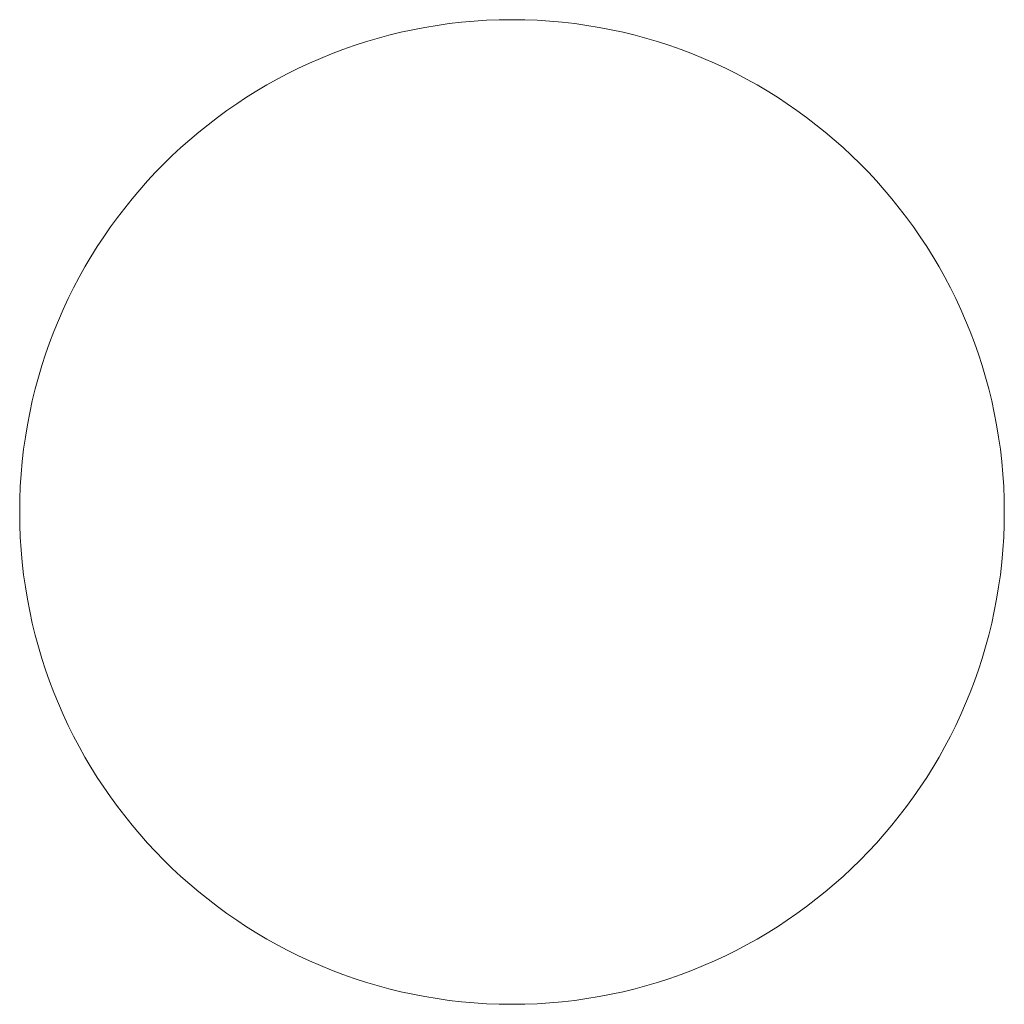
# Model space of a CAD drawing. Units: millimetres. Extents: x 1808 to 2221, y 1831 to 2244.
import ezdxf

# ---------------------------------------------------------------- set-up
doc = ezdxf.new("R2010")
doc.units = ezdxf.units.MM
doc.layers.add('M-CONS', color=8, linetype='Continuous', lineweight=13)

msp = doc.modelspace()

# ---------------------------------------------------------------- linework, layer by layer
at = {"layer": 'M-CONS'}
msp.add_circle((2014.67, 2037.65, 3), 206.68, dxfattribs=at)

doc.saveas('drawing.dxf')
